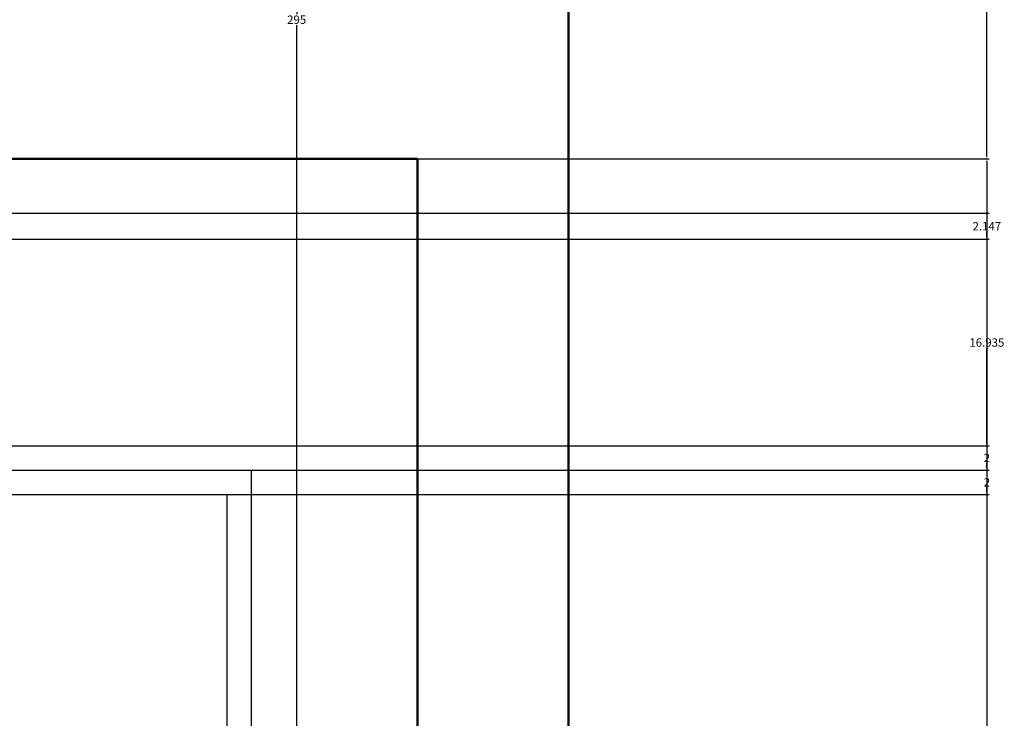
# Model space of a CAD drawing. Units: inches. Extents: x -139 to 346, y 72 to 413.
# Tile 14 of 18: x 265 to 346, y 185 to 242. Entities that reach past the tile are written whole.
import ezdxf

# ---------------------------------------------------------------- set-up
doc = ezdxf.new("R2010")
doc.units = ezdxf.units.IN
doc.header["$MEASUREMENT"] = 0
for name, color, linetype, lineweight in [('A-ANNO-DIMS', 2, 'Continuous', 18), ('A-DOOR', 3, 'Continuous', 25), ('A-WALL', 7, 'Continuous', 50)]:
    doc.layers.add(name, color=color, linetype=linetype, lineweight=lineweight)
doc.styles.get("Standard").update_dxf_attribs({"font": 'arial.ttf'})
doc.dimstyles.get("Standard").update_dxf_attribs({"dimtxt": 0.6875, "dimasz": 0.18, "dimexe": 0.18, "dimexo": 0.0625, "dimgap": 0.09, "dimtad": 0, "dimtih": 1, "dimtoh": 1, "dimdec": 4, "dimzin": 0, "dimdsep": 46, "dimlunit": 4, "dimtxsty": 'Standard', "dimcen": 0.09, "dimadec": 0, "dimazin": 0, "dimtfac": 1, "dimtdec": 4, "dimtofl": 0, "dimtmove": 0, "dimatfit": 3, "dimfxl": 1, "dimtolj": 1, "dimtzin": 0, "dimarcsym": 0})

# ---------------------------------------------------------------- blocks, each defined once
blk = doc.blocks.new('*D31')
at = {"layer": 'A-ANNO-DIMS', "color": 0, "lineweight": -2, "transparency": 16777216}
for p, q in [((309.827, 389.975), (287.409, 389.975)), ((287.589, 389.795), (287.589, 242.916)), ((287.589, 95.155), (287.589, 242.034)), ((309.827, 94.975), (287.409, 94.975))]:
    blk.add_line(p, q, dxfattribs=at)
at = {"layer": 'A-ANNO-DIMS', "color": 0, "transparency": 16777216}
for points in [[(287.559, 389.795), (287.619, 389.795), (287.589, 389.975)], [(287.559, 95.155), (287.619, 95.155), (287.589, 94.975)]]:
    blk.add_solid(points, dxfattribs=at)
at = {"layer": 'Defpoints', "color": 0, "transparency": 16777216}
for p in [(287.589, 389.975), (309.889, 389.975), (309.889, 94.975)]:
    blk.add_point(p, dxfattribs=at)
at = {"layer": 'A-ANNO-DIMS', "color": 0, "transparency": 16777216, "insert": (287.589, 242.475), "char_height": 0.6875, "attachment_point": 5}
blk.add_mtext('\\A1;295', dxfattribs=at)
blk = doc.blocks.new('*D33')
at = {"layer": 'A-ANNO-DIMS', "color": 0, "lineweight": -2, "transparency": 16777216}
for p, q in [((297.564, 231.061), (344.386, 231.061)), ((344.206, 230.881), (344.206, 172.273)), ((344.206, 112.784), (344.206, 171.391)), ((309.952, 112.604), (344.386, 112.604))]:
    blk.add_line(p, q, dxfattribs=at)
at = {"layer": 'A-ANNO-DIMS', "color": 0, "transparency": 16777216}
for points in [[(344.176, 230.881), (344.236, 230.881), (344.206, 231.061)], [(344.176, 112.784), (344.236, 112.784), (344.206, 112.604)]]:
    blk.add_solid(points, dxfattribs=at)
at = {"layer": 'Defpoints', "color": 0, "transparency": 16777216}
for p in [(297.501, 231.061), (344.206, 231.061), (309.889, 112.604)]:
    blk.add_point(p, dxfattribs=at)
at = {"layer": 'A-ANNO-DIMS', "color": 0, "transparency": 16777216, "insert": (344.206, 171.832), "char_height": 0.6875, "attachment_point": 5}
blk.add_mtext('\\A1;118.46', dxfattribs=at)
blk = doc.blocks.new('*D34')
at = {"layer": 'A-ANNO-DIMS', "color": 0, "lineweight": -2, "transparency": 16777216}
for p, q in [((274.309, 303.94), (344.386, 303.94)), ((344.206, 303.76), (344.206, 267.941)), ((344.206, 231.241), (344.206, 267.059)), ((297.564, 231.061), (344.386, 231.061))]:
    blk.add_line(p, q, dxfattribs=at)
at = {"layer": 'A-ANNO-DIMS', "color": 0, "transparency": 16777216}
for points in [[(344.176, 303.76), (344.236, 303.76), (344.206, 303.94)], [(344.176, 231.241), (344.236, 231.241), (344.206, 231.061)]]:
    blk.add_solid(points, dxfattribs=at)
at = {"layer": 'Defpoints', "color": 0, "transparency": 16777216}
for p in [(274.247, 303.94), (344.206, 303.94), (297.501, 231.061)]:
    blk.add_point(p, dxfattribs=at)
at = {"layer": 'A-ANNO-DIMS', "color": 0, "transparency": 16777216, "insert": (344.206, 267.5), "char_height": 0.6875, "attachment_point": 5}
blk.add_mtext('\\A1;72.88', dxfattribs=at)
blk = doc.blocks.new('*D54')
at = {"layer": 'A-ANNO-DIMS', "color": 0, "lineweight": -2, "transparency": 16777216}
for p, q in [((-47.211, 224.459), (344.386, 224.459)), ((344.206, 224.279), (344.206, 216.433)), ((344.206, 207.704), (344.206, 215.55)), ((-47.211, 207.524), (344.386, 207.524))]:
    blk.add_line(p, q, dxfattribs=at)
at = {"layer": 'A-ANNO-DIMS', "color": 0, "transparency": 16777216}
for points in [[(344.176, 224.279), (344.236, 224.279), (344.206, 224.459)], [(344.176, 207.704), (344.236, 207.704), (344.206, 207.524)]]:
    blk.add_solid(points, dxfattribs=at)
at = {"layer": 'Defpoints', "color": 0, "transparency": 16777216}
for p in [(-47.273, 224.459), (344.206, 224.459), (-47.273, 207.524)]:
    blk.add_point(p, dxfattribs=at)
at = {"layer": 'A-ANNO-DIMS', "color": 0, "transparency": 16777216, "insert": (344.206, 215.992), "char_height": 0.6875, "attachment_point": 5}
blk.add_mtext('\\A1;16.935', dxfattribs=at)
blk = doc.blocks.new('*D55')
at = {"layer": 'A-ANNO-DIMS', "color": 0, "lineweight": -2, "transparency": 16777216}
for p, q in [((-47.211, 226.606), (344.386, 226.606)), ((344.206, 226.426), (344.206, 225.968)), ((344.206, 224.639), (344.206, 225.097)), ((-47.211, 224.459), (344.386, 224.459))]:
    blk.add_line(p, q, dxfattribs=at)
at = {"layer": 'A-ANNO-DIMS', "color": 0, "transparency": 16777216}
for points in [[(344.176, 226.426), (344.236, 226.426), (344.206, 226.606)], [(344.176, 224.639), (344.236, 224.639), (344.206, 224.459)]]:
    blk.add_solid(points, dxfattribs=at)
at = {"layer": 'Defpoints', "color": 0, "transparency": 16777216}
for p in [(-47.273, 226.606), (344.206, 226.606), (-47.273, 224.459)]:
    blk.add_point(p, dxfattribs=at)
at = {"layer": 'A-ANNO-DIMS', "color": 0, "transparency": 16777216, "insert": (344.206, 225.533), "char_height": 0.6875, "attachment_point": 5}
blk.add_mtext('\\A1;2.147', dxfattribs=at)
blk = doc.blocks.new('*D65')
at = {"layer": 'A-ANNO-DIMS', "color": 0, "lineweight": -2, "transparency": 16777216}
for p, q in [((55.328, 205.524), (344.386, 205.524)), ((344.206, 205.344), (344.206, 178.581)), ((344.206, 150.938), (344.206, 177.701)), ((55.328, 150.758), (344.386, 150.758))]:
    blk.add_line(p, q, dxfattribs=at)
at = {"layer": 'A-ANNO-DIMS', "color": 0, "transparency": 16777216}
for points in [[(344.176, 205.344), (344.236, 205.344), (344.206, 205.524)], [(344.176, 150.938), (344.236, 150.938), (344.206, 150.758)]]:
    blk.add_solid(points, dxfattribs=at)
at = {"layer": 'Defpoints', "color": 0, "transparency": 16777216}
for p in [(55.265, 205.524), (344.206, 205.524), (55.265, 150.758)]:
    blk.add_point(p, dxfattribs=at)
at = {"layer": 'A-ANNO-DIMS', "color": 0, "transparency": 16777216, "insert": (344.206, 178.141), "char_height": 0.6875, "attachment_point": 5}
blk.add_mtext('\\A1;54.77', dxfattribs=at)
blk = doc.blocks.new('*D66')
at = {"layer": 'A-ANNO-DIMS', "color": 0, "lineweight": -2, "transparency": 16777216}
for p, q in [((57.328, 207.524), (344.386, 207.524)), ((344.206, 207.344), (344.206, 206.96)), ((344.206, 205.704), (344.206, 206.089)), ((55.328, 205.524), (344.386, 205.524))]:
    blk.add_line(p, q, dxfattribs=at)
at = {"layer": 'A-ANNO-DIMS', "color": 0, "transparency": 16777216}
for points in [[(344.176, 207.344), (344.236, 207.344), (344.206, 207.524)], [(344.176, 205.704), (344.236, 205.704), (344.206, 205.524)]]:
    blk.add_solid(points, dxfattribs=at)
at = {"layer": 'Defpoints', "color": 0, "transparency": 16777216}
for p in [(57.265, 207.524), (344.206, 207.524), (55.265, 205.524)]:
    blk.add_point(p, dxfattribs=at)
at = {"layer": 'A-ANNO-DIMS', "color": 0, "transparency": 16777216, "insert": (344.206, 206.524), "char_height": 0.6875, "attachment_point": 5}
blk.add_mtext('\\A1;2', dxfattribs=at)
blk = doc.blocks.new('*D67')
at = {"layer": 'A-ANNO-DIMS', "color": 0, "lineweight": -2, "transparency": 16777216}
for p, q in [((57.328, 207.524), (344.386, 207.524)), ((344.206, 207.344), (344.206, 165.091)), ((344.206, 121.955), (344.206, 164.209)), ((57.328, 121.775), (344.386, 121.775))]:
    blk.add_line(p, q, dxfattribs=at)
at = {"layer": 'A-ANNO-DIMS', "color": 0, "transparency": 16777216}
for points in [[(344.176, 207.344), (344.236, 207.344), (344.206, 207.524)], [(344.176, 121.955), (344.236, 121.955), (344.206, 121.775)]]:
    blk.add_solid(points, dxfattribs=at)
at = {"layer": 'Defpoints', "color": 0, "transparency": 16777216}
for p in [(57.265, 207.524), (344.206, 207.524), (57.265, 121.775)]:
    blk.add_point(p, dxfattribs=at)
at = {"layer": 'A-ANNO-DIMS', "color": 0, "transparency": 16777216, "insert": (344.206, 164.65), "char_height": 0.6875, "attachment_point": 5}
blk.add_mtext('\\A1;85.75', dxfattribs=at)
blk = doc.blocks.new('*D74')
at = {"layer": 'A-ANNO-DIMS', "color": 0, "lineweight": -2, "transparency": 16777216}
for p, q in [((283.912, 205.524), (344.386, 205.524)), ((344.206, 205.344), (344.206, 155.475)), ((344.206, 104.723), (344.206, 154.593)), ((283.912, 104.543), (344.386, 104.543))]:
    blk.add_line(p, q, dxfattribs=at)
at = {"layer": 'A-ANNO-DIMS', "color": 0, "transparency": 16777216}
for points in [[(344.176, 205.344), (344.236, 205.344), (344.206, 205.524)], [(344.176, 104.723), (344.236, 104.723), (344.206, 104.543)]]:
    blk.add_solid(points, dxfattribs=at)
at = {"layer": 'Defpoints', "color": 0, "transparency": 16777216}
for p in [(283.85, 205.524), (344.206, 205.524), (283.85, 104.543)]:
    blk.add_point(p, dxfattribs=at)
at = {"layer": 'A-ANNO-DIMS', "color": 0, "transparency": 16777216, "insert": (344.206, 155.034), "char_height": 0.6875, "attachment_point": 5}
blk.add_mtext('\\A1;100.98', dxfattribs=at)
blk = doc.blocks.new('*D78')
at = {"layer": 'A-ANNO-DIMS', "color": 0, "lineweight": -2, "transparency": 16777216}
for p, q in [((281.912, 203.524), (344.386, 203.524)), ((344.206, 203.344), (344.206, 176.724)), ((344.206, 149.221), (344.206, 175.842)), ((280.266, 149.041), (344.386, 149.041))]:
    blk.add_line(p, q, dxfattribs=at)
at = {"layer": 'A-ANNO-DIMS', "color": 0, "transparency": 16777216}
for points in [[(344.176, 203.344), (344.236, 203.344), (344.206, 203.524)], [(344.176, 149.221), (344.236, 149.221), (344.206, 149.041)]]:
    blk.add_solid(points, dxfattribs=at)
at = {"layer": 'Defpoints', "color": 0, "transparency": 16777216}
for p in [(281.85, 203.524), (344.206, 203.524), (280.204, 149.041)]:
    blk.add_point(p, dxfattribs=at)
at = {"layer": 'A-ANNO-DIMS', "color": 0, "transparency": 16777216, "insert": (344.206, 176.283), "char_height": 0.6875, "attachment_point": 5}
blk.add_mtext('\\A1;54.48', dxfattribs=at)
blk = doc.blocks.new('*D79')
at = {"layer": 'A-ANNO-DIMS', "color": 0, "lineweight": -2, "transparency": 16777216}
for p, q in [((283.912, 205.524), (344.386, 205.524)), ((344.206, 205.344), (344.206, 204.96)), ((344.206, 203.704), (344.206, 204.089)), ((281.912, 203.524), (344.386, 203.524))]:
    blk.add_line(p, q, dxfattribs=at)
at = {"layer": 'A-ANNO-DIMS', "color": 0, "transparency": 16777216}
for points in [[(344.176, 205.344), (344.236, 205.344), (344.206, 205.524)], [(344.176, 203.704), (344.236, 203.704), (344.206, 203.524)]]:
    blk.add_solid(points, dxfattribs=at)
at = {"layer": 'Defpoints', "color": 0, "transparency": 16777216}
for p in [(283.85, 205.524), (344.206, 205.524), (281.85, 203.524)]:
    blk.add_point(p, dxfattribs=at)
at = {"layer": 'A-ANNO-DIMS', "color": 0, "transparency": 16777216, "insert": (344.206, 204.524), "char_height": 0.6875, "attachment_point": 5}
blk.add_mtext('\\A1;2', dxfattribs=at)
blk = doc.blocks.new('*D86')
at = {"layer": 'A-ANNO-DIMS', "color": 0, "lineweight": -2, "transparency": 16777216}
for p, q in [((281.85, 203.462), (281.85, 72.495)), ((279.438, 148.978), (279.438, 72.495)), ((279.618, 72.675), (279.721, 72.675)), ((281.67, 72.675), (281.566, 72.675))]:
    blk.add_line(p, q, dxfattribs=at)
at = {"layer": 'A-ANNO-DIMS', "color": 0, "transparency": 16777216}
for points in [[(279.618, 72.705), (279.618, 72.645), (279.438, 72.675)], [(281.67, 72.705), (281.67, 72.645), (281.85, 72.675)]]:
    blk.add_solid(points, dxfattribs=at)
at = {"layer": 'Defpoints', "color": 0, "transparency": 16777216}
for p in [(281.85, 203.524), (279.438, 149.041), (281.85, 72.675)]:
    blk.add_point(p, dxfattribs=at)
at = {"layer": 'A-ANNO-DIMS', "color": 0, "transparency": 16777216, "insert": (280.644, 72.675), "char_height": 0.6875, "attachment_point": 5}
blk.add_mtext('\\A1;2.41', dxfattribs=at)

msp = doc.modelspace()

# ---------------------------------------------------------------- linework, layer by layer
at = {"layer": 'A-DOOR'}
for points in [[(229.972, 205.5243), (283.8497, 205.5243), (283.8497, 104.5429), (229.972, 104.5429)], [(231.972, 203.5243), (281.8497, 203.5243), (281.8497, 106.5429), (231.972, 106.5429)]]:
    msp.add_lwpolyline(points, close=True, dxfattribs=at)
at = {"layer": 'A-WALL'}
for p, q in [((309.8894, 94.9748), (309.8894, 382.9748)), ((297.5013, 231.0607), (112.6506, 231.0607)), ((297.5013, 94.9748), (297.5013, 231.0607))]:
    msp.add_line(p, q, dxfattribs=at)

# ---------------------------------------------------------------- dimensions: what is measured, and where the dimension line sits
at = {"layer": 'A-ANNO-DIMS'}
for base, p1, p2, override, picture, middle in [((287.5894, 389.9748), (309.8894, 94.9748), (309.8894, 389.9748), {"dimdec": 0, "dimlfac": 1, "dimrnd": 0, "dimzin": 0, "dimdsep": 46, "dimlunit": 2}, '*D31', (287.5894, 242.4748)), ((344.2055, 303.9402), (297.5013, 231.0607), (274.2465, 303.9402), {"dimdec": 2, "dimlfac": 1, "dimrnd": 0, "dimzin": 0, "dimdsep": 46, "dimlunit": 2}, '*D34', (344.2055, 267.5005)), ((344.2055, 231.0607), (309.8894, 112.6042), (297.5013, 231.0607), {"dimdec": 2, "dimlfac": 1, "dimrnd": 0, "dimzin": 0, "dimdsep": 46, "dimlunit": 2}, '*D33', (344.2055, 171.8325)), ((344.2055, 226.6062), (-47.2734, 224.4591), (-47.2734, 226.6062), {"dimdec": 3, "dimlfac": 1, "dimrnd": 0, "dimzin": 0, "dimdsep": 46, "dimlunit": 2}, '*D55', (344.2055, 225.5327)), ((344.2055, 224.4591), (-47.2734, 207.5243), (-47.2734, 224.4591), {"dimdec": 3, "dimlfac": 1, "dimrnd": 0, "dimzin": 0, "dimdsep": 46, "dimlunit": 2}, '*D54', (344.2055, 215.9917)), ((344.2055, 207.5243), (55.2654, 205.5243), (57.2654, 207.5243), {"dimdec": 0, "dimlfac": 1, "dimrnd": 0, "dimzin": 0, "dimdsep": 46, "dimlunit": 2}, '*D66', (344.2055, 206.5243)), ((344.2055, 207.5243), (57.2654, 121.7753), (57.2654, 207.5243), {"dimdec": 2, "dimlfac": 1, "dimrnd": 0, "dimzin": 0, "dimdsep": 46, "dimlunit": 2}, '*D67', (344.2055, 164.6498)), ((344.2055, 205.5243), (55.2654, 150.7576), (55.2654, 205.5243), {"dimdec": 2, "dimlfac": 1, "dimrnd": 0, "dimzin": 0, "dimdsep": 46, "dimlunit": 2}, '*D65', (344.2055, 178.141)), ((344.2055, 205.5243), (281.8497, 203.5243), (283.8497, 205.5243), {"dimdec": 0, "dimlfac": 1, "dimrnd": 0, "dimzin": 0, "dimdsep": 46, "dimlunit": 2}, '*D79', (344.2055, 204.5243)), ((344.2055, 205.5243), (283.8497, 104.5429), (283.8497, 205.5243), {"dimdec": 2, "dimlfac": 1, "dimrnd": 0, "dimzin": 0, "dimdsep": 46, "dimlunit": 2}, '*D74', (344.2055, 155.0336)), ((344.2055, 203.5243), (280.2036, 149.0409), (281.8497, 203.5243), {"dimdec": 2, "dimlfac": 1, "dimrnd": 0, "dimzin": 0, "dimdsep": 46, "dimlunit": 2}, '*D78', (344.2055, 176.2826))]:
    dim = msp.add_linear_dim(base=base, p1=p1, p2=p2, angle=90, dimstyle='Standard', override=override, dxfattribs=at)
    dim.commit()
    dim.dimension.update_dxf_attribs({"geometry": picture, "text_midpoint": middle})
dim = msp.add_linear_dim(base=(281.8497, 72.6748), p1=(279.438, 149.0409), p2=(281.8497, 203.5243), dimstyle='Standard', override={"dimdec": 2, "dimlfac": 1, "dimrnd": 0, "dimzin": 0, "dimdsep": 46, "dimlunit": 2}, dxfattribs=at)
dim.commit()
dim.dimension.update_dxf_attribs({"geometry": '*D86', "text_midpoint": (280.6438, 72.6748)})

doc.saveas('drawing.dxf')
